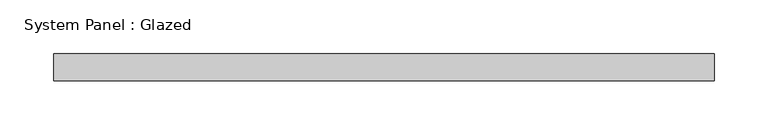
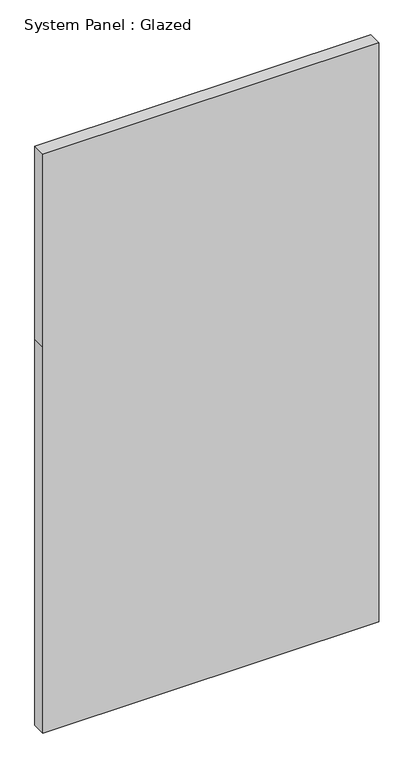
"""IFC4 building model written with IfcOpenShell, lengths in millimetres: plate geometry, System Panel : Glazed."""

from ifc_helpers import new_model, si_unit, frame, origin, place, context, project, spatial, polyline, outline, extrude, source, transform, mapped, element, save


def system_panel_glazed_5a74f323(model_context):
    return source(origin(), model_context, "Body", "SweptSolid", [
        extrude(outline(polyline([(0.0, -307.975), (0.0, 307.975), (747.9673296, 307.975), (1121.9509944, 307.975), (1121.9509944, -307.975), (747.9673296, -307.975), (0.0, -307.975)])), frame((0.0, 19.05, 0.0), z_axis=(0.0, 1.0, 0.0), x_axis=(0.0, 0.0, 1.0)), (0.0, 0.0, 1.0), 25.4),
    ])


if __name__ == "__main__":
    model = new_model("IFC4")
    model_context = context("Model", 3, world=origin())
    ifc_project = project(units=[si_unit("LENGTHUNIT", "METRE", prefix="MILLI")], contexts=[model_context])
    site = spatial("IfcSite", under=ifc_project)
    building = spatial("IfcBuilding", under=site)
    placement = place(None, origin())
    system_panel_glazed_shape = system_panel_glazed_5a74f323(model_context)
    element("IfcPlate", 1, ObjectType="System Panel : Glazed", at=placement, inside=building, context=model_context, shape_type="MappedRepresentation", body=[
        mapped(system_panel_glazed_shape, transform((0.0, 0.0, 0.0), x_axis=(1.0, 0.0, 0.0), y_axis=(0.0, 1.0, 0.0), z_axis=(0.0, 0.0, 1.0))),
    ])
    save(model, "model.ifc")

# Revit data of these elements
# Type "System Panel : Glazed"
#   Construction Type Id = "GSP4R"
#   Analytic Construction = "1/8 in Pilkington single glazing"
#   Visual Light Transmittance = 0.9
#   Solar Heat Gain Coefficient = 0.86
#   Heat Transfer Coefficient (U) = 1.18115 BTU/(h·ft²·°F)
#   Define Thermal Properties by = 1
# Element 1 (IfcPlate, "System Panel : Glazed")
#   Materials on its faces: "Glass"
# Materials
#   "Glass": class "Glass", colour RGB 0 128 192, transparency 0.75, Description = "Soda Lime Glass", Cost = 0
